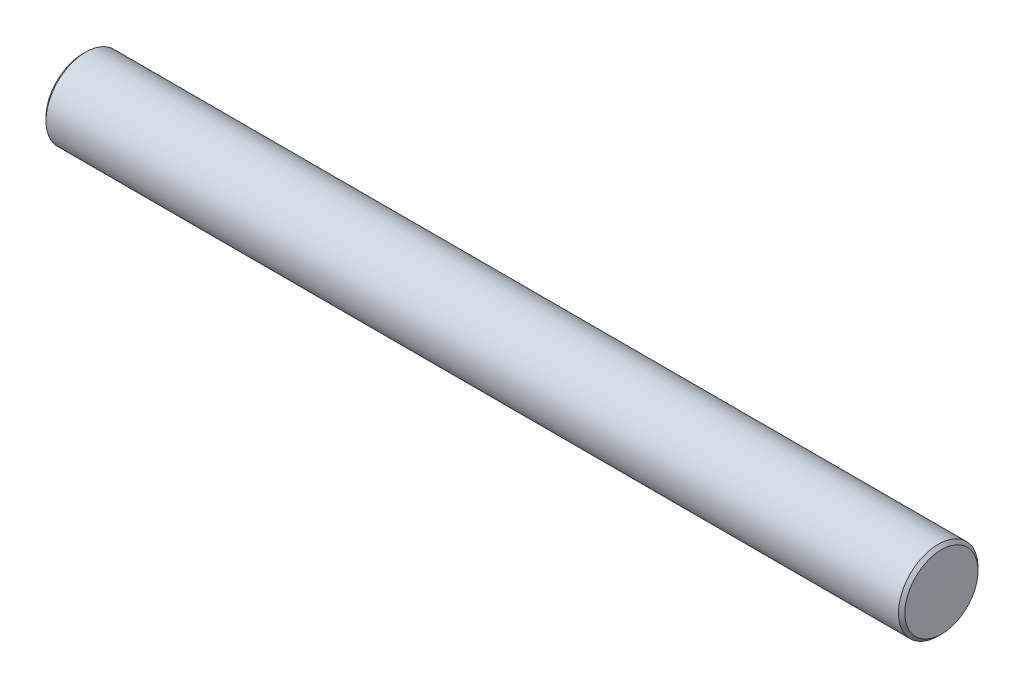
ISO-10303-21;
HEADER;
FILE_DESCRIPTION(('STEP AP214'),'2;1');
FILE_NAME('part.step','',(''),(''),'','','');
FILE_SCHEMA(('AUTOMOTIVE_DESIGN { 1 0 10303 214 1 1 1 1 }'));
ENDSEC;
DATA;
#1=APPLICATION_CONTEXT('core data for automotive mechanical design processes');
#2=APPLICATION_PROTOCOL_DEFINITION('international standard','automotive_design',2000,#1);
#3=PRODUCT_CONTEXT('',#1,'mechanical');
#4=PRODUCT('Part','Part','',(#3));
#5=PRODUCT_RELATED_PRODUCT_CATEGORY('part','',(#4));
#6=PRODUCT_DEFINITION_FORMATION('','',#4);
#7=PRODUCT_DEFINITION_CONTEXT('part definition',#1,'design');
#8=PRODUCT_DEFINITION('design','',#6,#7);
#9=PRODUCT_DEFINITION_SHAPE('','',#8);
#10=(LENGTH_UNIT() NAMED_UNIT(*) SI_UNIT(.MILLI.,.METRE.));
#11=(NAMED_UNIT(*) PLANE_ANGLE_UNIT() SI_UNIT($,.RADIAN.));
#12=(NAMED_UNIT(*) SI_UNIT($,.STERADIAN.) SOLID_ANGLE_UNIT());
#13=UNCERTAINTY_MEASURE_WITH_UNIT(LENGTH_MEASURE(1.E-05),#10,'distance_accuracy_value','');
#14=(GEOMETRIC_REPRESENTATION_CONTEXT(3) GLOBAL_UNCERTAINTY_ASSIGNED_CONTEXT((#13)) GLOBAL_UNIT_ASSIGNED_CONTEXT((#10,
#11,#12)) REPRESENTATION_CONTEXT('',''));
#15=CARTESIAN_POINT('',(0.,0.,0.));
#16=DIRECTION('',(0.,0.,1.));
#17=DIRECTION('',(1.,0.,0.));
#18=AXIS2_PLACEMENT_3D('',#15,#16,#17);
#19=CARTESIAN_POINT('',(270.,25.,0.));
#20=DIRECTION('',(-1.,0.,0.));
#21=DIRECTION('',(0.,-1.,0.));
#22=AXIS2_PLACEMENT_3D('',#19,#20,#21);
#23=PLANE('',#22);
#24=CARTESIAN_POINT('',(270.,0.,0.));
#25=DIRECTION('',(-1.,0.,0.));
#26=DIRECTION('',(0.,-1.,0.));
#27=AXIS2_PLACEMENT_3D('',#24,#25,#26);
#28=CIRCLE('',#27,23.0000000000001);
#29=CARTESIAN_POINT('',(270.,-23.0000000000001,0.));
#30=VERTEX_POINT('',#29);
#31=EDGE_CURVE('E10',#30,#30,#28,.F.);
#32=ORIENTED_EDGE('',*,*,#31,.T.);
#33=EDGE_LOOP('',(#32));
#34=FACE_BOUND('',#33,.T.);
#35=ADVANCED_FACE('F39',(#34),#23,.F.);
#36=CARTESIAN_POINT('',(-270.,0.,0.));
#37=DIRECTION('',(-1.,0.,0.));
#38=DIRECTION('',(0.,-1.,0.));
#39=AXIS2_PLACEMENT_3D('',#36,#37,#38);
#40=CYLINDRICAL_SURFACE('',#39,25.);
#41=CARTESIAN_POINT('',(-268.,0.,0.));
#42=DIRECTION('',(1.,0.,0.));
#43=DIRECTION('',(0.,1.,0.));
#44=AXIS2_PLACEMENT_3D('',#41,#42,#43);
#45=CIRCLE('',#44,25.);
#46=CARTESIAN_POINT('',(-268.,25.,0.));
#47=VERTEX_POINT('',#46);
#48=EDGE_CURVE('E50',#47,#47,#45,.T.);
#49=ORIENTED_EDGE('',*,*,#48,.T.);
#50=EDGE_LOOP('',(#49));
#51=FACE_BOUND('',#50,.T.);
#52=CARTESIAN_POINT('',(268.,0.,0.));
#53=DIRECTION('',(-1.,0.,0.));
#54=DIRECTION('',(0.,-1.,0.));
#55=AXIS2_PLACEMENT_3D('',#52,#53,#54);
#56=CIRCLE('',#55,25.);
#57=CARTESIAN_POINT('',(268.,-25.,0.));
#58=VERTEX_POINT('',#57);
#59=EDGE_CURVE('E51',#58,#58,#56,.T.);
#60=ORIENTED_EDGE('',*,*,#59,.T.);
#61=EDGE_LOOP('',(#60));
#62=FACE_BOUND('',#61,.T.);
#63=ADVANCED_FACE('F72',(#51,#62),#40,.T.);
#64=CARTESIAN_POINT('',(-270.,24.9999999999999,0.));
#65=DIRECTION('',(1.,0.,0.));
#66=DIRECTION('',(0.,1.,0.));
#67=AXIS2_PLACEMENT_3D('',#64,#65,#66);
#68=PLANE('',#67);
#69=CARTESIAN_POINT('',(-270.,0.,0.));
#70=DIRECTION('',(1.,0.,0.));
#71=DIRECTION('',(0.,1.,0.));
#72=AXIS2_PLACEMENT_3D('',#69,#70,#71);
#73=CIRCLE('',#72,22.9999999999997);
#74=CARTESIAN_POINT('',(-270.,22.9999999999997,0.));
#75=VERTEX_POINT('',#74);
#76=EDGE_CURVE('E54',#75,#75,#73,.F.);
#77=ORIENTED_EDGE('',*,*,#76,.T.);
#78=EDGE_LOOP('',(#77));
#79=FACE_BOUND('',#78,.T.);
#80=ADVANCED_FACE('F63',(#79),#68,.F.);
#81=CARTESIAN_POINT('',(-270.,0.,0.));
#82=DIRECTION('',(1.,0.,0.));
#83=DIRECTION('',(0.,1.,0.));
#84=AXIS2_PLACEMENT_3D('',#81,#82,#83);
#85=CONICAL_SURFACE('',#84,22.9999999999997,0.785398163397453);
#86=ORIENTED_EDGE('',*,*,#48,.F.);
#87=EDGE_LOOP('',(#86));
#88=FACE_BOUND('',#87,.T.);
#89=ORIENTED_EDGE('',*,*,#76,.F.);
#90=EDGE_LOOP('',(#89));
#91=FACE_BOUND('',#90,.T.);
#92=ADVANCED_FACE('F61',(#88,#91),#85,.T.);
#93=CARTESIAN_POINT('',(268.,0.,0.));
#94=DIRECTION('',(-1.,0.,0.));
#95=DIRECTION('',(0.,-1.,0.));
#96=AXIS2_PLACEMENT_3D('',#93,#94,#95);
#97=CONICAL_SURFACE('',#96,25.,0.785398163397466);
#98=ORIENTED_EDGE('',*,*,#31,.F.);
#99=EDGE_LOOP('',(#98));
#100=FACE_BOUND('',#99,.T.);
#101=ORIENTED_EDGE('',*,*,#59,.F.);
#102=EDGE_LOOP('',(#101));
#103=FACE_BOUND('',#102,.T.);
#104=ADVANCED_FACE('F45',(#100,#103),#97,.T.);
#105=CLOSED_SHELL('',(#35,#63,#80,#92,#104));
#106=MANIFOLD_SOLID_BREP('B2',#105);
#107=ADVANCED_BREP_SHAPE_REPRESENTATION('',(#18,#106),#14);
#108=SHAPE_DEFINITION_REPRESENTATION(#9,#107);
ENDSEC;
END-ISO-10303-21;
